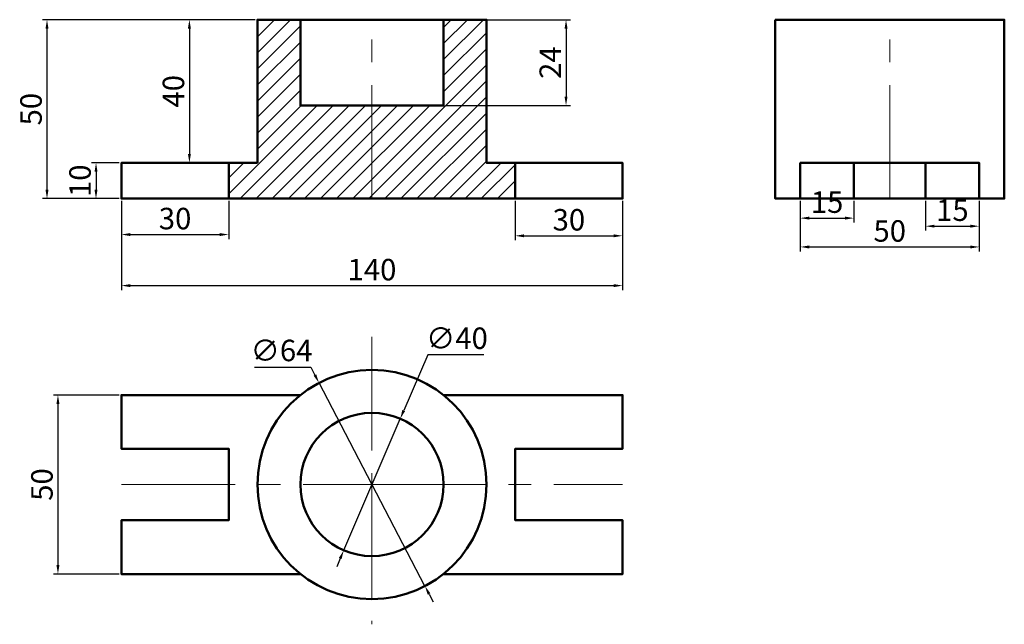
# Model space of a CAD drawing. Units: millimetres. Extents: x 177 to 452, y 51 to 220.
import ezdxf

# ---------------------------------------------------------------- set-up
doc = ezdxf.new("R2010")
doc.units = ezdxf.units.MM
doc.linetypes.add('CENTER', pattern=[50.8, 31.75, -6.35, 6.35, -6.35])
for name, color, linetype, lineweight in [('M-CNTR', 1, 'CENTER', 18), ('M-DIMS', 2, 'Continuous', 25), ('M-HATC', 8, 'Continuous', 18), ('M-OUTL', 7, 'Continuous', 50)]:
    doc.layers.add(name, color=color, linetype=linetype, lineweight=lineweight)
doc.styles.get("Standard").update_dxf_attribs({"font": 'arial.ttf'})
doc.dimstyles.new('ISO-25', dxfattribs={"dimtxt": 6, "dimasz": 2.5, "dimexe": 1.25, "dimexo": 0.625, "dimtad": 1, "dimtoh": 1, "dimdec": 1, "dimtxsty": 'Standard', "dimcen": 2.5, "dimadec": 0, "dimazin": 0, "dimtfac": 1, "dimtdec": 1, "dimtmove": 0, "dimatfit": 3, "dimfxl": 1, "dimarcsym": 0})

# ---------------------------------------------------------------- blocks, each defined once
blk = doc.blocks.new('*D1')
at = {"layer": 'Defpoints', "color": 0, "transparency": 16777216}
for p in [(295.75, 220.14), (295.75, 196.14), (329.95, 196.14)]:
    blk.add_point(p, dxfattribs=at)
at = {"layer": 'M-DIMS', "color": 0, "lineweight": -2, "transparency": 16777216}
for p, q in [((296.38, 220.14), (331.2, 220.14)), ((329.95, 217.64), (329.95, 198.64)), ((296.38, 196.14), (331.2, 196.14))]:
    blk.add_line(p, q, dxfattribs=at)
at = {"layer": 'M-DIMS', "color": 0, "transparency": 16777216}
for points in [[(329.54, 217.64), (330.37, 217.64), (329.95, 220.14)], [(329.54, 198.64), (330.37, 198.64), (329.95, 196.14)]]:
    blk.add_solid(points, dxfattribs=at)
at = {"layer": 'M-DIMS', "color": 0, "transparency": 16777216, "insert": (326.32, 208.14), "char_height": 6, "attachment_point": 5, "rotation": 90}
blk.add_mtext('24', dxfattribs=at)
blk = doc.blocks.new('*D2')
at = {"layer": 'Defpoints', "color": 0, "transparency": 16777216}
for p in [(205.75, 170.14), (235.75, 170.14), (235.75, 160.11)]:
    blk.add_point(p, dxfattribs=at)
at = {"layer": 'M-DIMS', "color": 0, "lineweight": -2, "transparency": 16777216}
for p, q in [((205.75, 169.51), (205.75, 158.86)), ((235.75, 169.51), (235.75, 158.86)), ((208.25, 160.11), (233.25, 160.11))]:
    blk.add_line(p, q, dxfattribs=at)
at = {"layer": 'M-DIMS', "color": 0, "transparency": 16777216}
for points in [[(208.25, 160.53), (208.25, 159.7), (205.75, 160.11)], [(233.25, 160.53), (233.25, 159.7), (235.75, 160.11)]]:
    blk.add_solid(points, dxfattribs=at)
at = {"layer": 'M-DIMS', "color": 0, "transparency": 16777216, "insert": (220.75, 163.8), "char_height": 6, "attachment_point": 5}
blk.add_mtext('30', dxfattribs=at)
blk = doc.blocks.new('*D3')
at = {"layer": 'Defpoints', "color": 0, "transparency": 16777216}
for p in [(315.75, 170.14), (345.75, 170.14), (345.75, 159.76)]:
    blk.add_point(p, dxfattribs=at)
at = {"layer": 'M-DIMS', "color": 0, "lineweight": -2, "transparency": 16777216}
for p, q in [((315.75, 169.51), (315.75, 158.51)), ((345.75, 169.51), (345.75, 158.51)), ((318.25, 159.76), (343.25, 159.76))]:
    blk.add_line(p, q, dxfattribs=at)
at = {"layer": 'M-DIMS', "color": 0, "transparency": 16777216}
for points in [[(318.25, 160.18), (318.25, 159.35), (315.75, 159.76)], [(343.25, 160.18), (343.25, 159.35), (345.75, 159.76)]]:
    blk.add_solid(points, dxfattribs=at)
at = {"layer": 'M-DIMS', "color": 0, "transparency": 16777216, "insert": (330.75, 163.46), "char_height": 6, "attachment_point": 5}
blk.add_mtext('30', dxfattribs=at)
blk = doc.blocks.new('*D4')
at = {"layer": 'Defpoints', "color": 0, "transparency": 16777216}
for p in [(205.75, 170.14), (345.75, 170.14), (345.75, 145.85)]:
    blk.add_point(p, dxfattribs=at)
at = {"layer": 'M-DIMS', "color": 0, "lineweight": -2, "transparency": 16777216}
for p, q in [((205.75, 169.51), (205.75, 144.6)), ((345.75, 169.51), (345.75, 144.6)), ((208.25, 145.85), (343.25, 145.85))]:
    blk.add_line(p, q, dxfattribs=at)
at = {"layer": 'M-DIMS', "color": 0, "transparency": 16777216}
for points in [[(208.25, 146.26), (208.25, 145.43), (205.75, 145.85)], [(343.25, 146.26), (343.25, 145.43), (345.75, 145.85)]]:
    blk.add_solid(points, dxfattribs=at)
at = {"layer": 'M-DIMS', "color": 0, "transparency": 16777216, "insert": (275.75, 149.53), "char_height": 6, "attachment_point": 5}
blk.add_mtext('140', dxfattribs=at)
blk = doc.blocks.new('*D5')
at = {"layer": 'Defpoints', "color": 0, "transparency": 16777216}
for p in [(205.75, 180.14), (198.67, 170.14), (205.75, 170.14)]:
    blk.add_point(p, dxfattribs=at)
at = {"layer": 'M-DIMS', "color": 0, "lineweight": -2, "transparency": 16777216}
for p, q in [((205.13, 180.14), (197.42, 180.14)), ((198.67, 177.64), (198.67, 172.64)), ((205.13, 170.14), (197.42, 170.14))]:
    blk.add_line(p, q, dxfattribs=at)
at = {"layer": 'M-DIMS', "color": 0, "transparency": 16777216}
for points in [[(198.25, 177.64), (199.08, 177.64), (198.67, 180.14)], [(198.25, 172.64), (199.08, 172.64), (198.67, 170.14)]]:
    blk.add_solid(points, dxfattribs=at)
at = {"layer": 'M-DIMS', "color": 0, "transparency": 16777216, "insert": (194.98, 175.14), "char_height": 6, "attachment_point": 5, "rotation": 90}
blk.add_mtext('10', dxfattribs=at)
blk = doc.blocks.new('*D6')
at = {"layer": 'Defpoints', "color": 0, "transparency": 16777216}
for p in [(243.75, 220.14), (224.75, 180.14), (243.75, 180.14)]:
    blk.add_point(p, dxfattribs=at)
at = {"layer": 'M-DIMS', "color": 0, "lineweight": -2, "transparency": 16777216}
for p, q in [((243.13, 220.14), (223.5, 220.14)), ((224.75, 217.64), (224.75, 182.64)), ((243.13, 180.14), (223.5, 180.14))]:
    blk.add_line(p, q, dxfattribs=at)
at = {"layer": 'M-DIMS', "color": 0, "transparency": 16777216}
for points in [[(224.34, 217.64), (225.17, 217.64), (224.75, 220.14)], [(224.34, 182.64), (225.17, 182.64), (224.75, 180.14)]]:
    blk.add_solid(points, dxfattribs=at)
at = {"layer": 'M-DIMS', "color": 0, "transparency": 16777216, "insert": (221.07, 200.14), "char_height": 6, "attachment_point": 5, "rotation": 90}
blk.add_mtext('40', dxfattribs=at)
blk = doc.blocks.new('*D7')
at = {"layer": 'Defpoints', "color": 0, "transparency": 16777216}
for p in [(243.75, 220.14), (184.97, 170.14), (205.75, 170.14)]:
    blk.add_point(p, dxfattribs=at)
at = {"layer": 'M-DIMS', "color": 0, "lineweight": -2, "transparency": 16777216}
for p, q in [((243.13, 220.14), (183.72, 220.14)), ((184.97, 217.64), (184.97, 172.64)), ((205.13, 170.14), (183.72, 170.14))]:
    blk.add_line(p, q, dxfattribs=at)
at = {"layer": 'M-DIMS', "color": 0, "transparency": 16777216}
for points in [[(184.56, 217.64), (185.39, 217.64), (184.97, 220.14)], [(184.56, 172.64), (185.39, 172.64), (184.97, 170.14)]]:
    blk.add_solid(points, dxfattribs=at)
at = {"layer": 'M-DIMS', "color": 0, "transparency": 16777216, "insert": (181.29, 195.14), "char_height": 6, "attachment_point": 5, "rotation": 90}
blk.add_mtext('50', dxfattribs=at)
blk = doc.blocks.new('*D8')
at = {"layer": 'Defpoints', "color": 0, "transparency": 16777216}
for p in [(395.37, 170.14), (445.37, 170.14), (445.37, 156.65)]:
    blk.add_point(p, dxfattribs=at)
at = {"layer": 'M-DIMS', "color": 0, "lineweight": -2, "transparency": 16777216}
for p, q in [((395.37, 169.51), (395.37, 155.4)), ((445.37, 169.51), (445.37, 155.4)), ((397.87, 156.65), (442.87, 156.65))]:
    blk.add_line(p, q, dxfattribs=at)
at = {"layer": 'M-DIMS', "color": 0, "transparency": 16777216}
for points in [[(397.87, 157.06), (397.87, 156.23), (395.37, 156.65)], [(442.87, 157.06), (442.87, 156.23), (445.37, 156.65)]]:
    blk.add_solid(points, dxfattribs=at)
at = {"layer": 'M-DIMS', "color": 0, "transparency": 16777216, "insert": (420.37, 160.34), "char_height": 6, "attachment_point": 5}
blk.add_mtext('50', dxfattribs=at)
blk = doc.blocks.new('*D9')
at = {"layer": 'Defpoints', "color": 0, "transparency": 16777216}
for p in [(395.37, 170.14), (410.37, 170.14), (410.37, 164.7)]:
    blk.add_point(p, dxfattribs=at)
at = {"layer": 'M-DIMS', "color": 0, "lineweight": -2, "transparency": 16777216}
for p, q in [((395.37, 169.51), (395.37, 163.45)), ((410.37, 169.51), (410.37, 163.45)), ((397.87, 164.7), (407.87, 164.7))]:
    blk.add_line(p, q, dxfattribs=at)
at = {"layer": 'M-DIMS', "color": 0, "transparency": 16777216}
for points in [[(397.87, 165.12), (397.87, 164.29), (395.37, 164.7)], [(407.87, 165.12), (407.87, 164.29), (410.37, 164.7)]]:
    blk.add_solid(points, dxfattribs=at)
at = {"layer": 'M-DIMS', "color": 0, "transparency": 16777216, "insert": (402.87, 168.39), "char_height": 6, "attachment_point": 5}
blk.add_mtext('15', dxfattribs=at)
blk = doc.blocks.new('*D10')
at = {"layer": 'Defpoints', "color": 0, "transparency": 16777216}
for p in [(430.37, 170.14), (445.37, 170.14), (445.37, 162.45)]:
    blk.add_point(p, dxfattribs=at)
at = {"layer": 'M-DIMS', "color": 0, "lineweight": -2, "transparency": 16777216}
for p, q in [((430.37, 169.51), (430.37, 161.2)), ((445.37, 169.51), (445.37, 161.2)), ((432.87, 162.45), (442.87, 162.45))]:
    blk.add_line(p, q, dxfattribs=at)
at = {"layer": 'M-DIMS', "color": 0, "transparency": 16777216}
for points in [[(432.87, 162.87), (432.87, 162.04), (430.37, 162.45)], [(442.87, 162.87), (442.87, 162.04), (445.37, 162.45)]]:
    blk.add_solid(points, dxfattribs=at)
at = {"layer": 'M-DIMS', "color": 0, "transparency": 16777216, "insert": (437.87, 166.14), "char_height": 6, "attachment_point": 5}
blk.add_mtext('15', dxfattribs=at)
blk = doc.blocks.new('*D11')
at = {"layer": 'Defpoints', "color": 0, "transparency": 16777216}
for p in [(260.96, 118.66), (290.55, 61.9)]:
    blk.add_point(p, dxfattribs=at)
at = {"layer": 'M-DIMS', "color": 0, "lineweight": -2, "transparency": 16777216}
for p, q in [((242.93, 123.09), (258.65, 123.09)), ((258.65, 123.09), (259.81, 120.87)), ((290.55, 61.9), (260.96, 118.66)), ((291.7, 59.69), (292.86, 57.47))]:
    blk.add_line(p, q, dxfattribs=at)
at = {"layer": 'M-DIMS', "color": 0, "transparency": 16777216}
for points in [[(260.18, 121.06), (259.44, 120.68), (260.96, 118.66)], [(292.07, 59.88), (291.33, 59.49), (290.55, 61.9)]]:
    blk.add_solid(points, dxfattribs=at)
at = {"layer": 'M-DIMS', "color": 0, "transparency": 16777216, "insert": (250.48, 126.95), "char_height": 6, "attachment_point": 5}
blk.add_mtext('∅64', dxfattribs=at)
blk = doc.blocks.new('*D12')
at = {"layer": 'Defpoints', "color": 0, "transparency": 16777216}
for p in [(283.64, 108.66), (267.87, 71.9)]:
    blk.add_point(p, dxfattribs=at)
at = {"layer": 'M-DIMS', "color": 0, "lineweight": -2, "transparency": 16777216}
for p, q in [((291.31, 126.52), (284.63, 110.96)), ((307.03, 126.52), (291.31, 126.52)), ((267.87, 71.9), (283.64, 108.66)), ((266.88, 69.6), (265.89, 67.31))]:
    blk.add_line(p, q, dxfattribs=at)
at = {"layer": 'M-DIMS', "color": 0, "transparency": 16777216}
for points in [[(284.24, 111.12), (285.01, 110.79), (283.64, 108.66)], [(266.5, 69.77), (267.26, 69.44), (267.87, 71.9)]]:
    blk.add_solid(points, dxfattribs=at)
at = {"layer": 'M-DIMS', "color": 0, "transparency": 16777216, "insert": (299.48, 130.37), "char_height": 6, "attachment_point": 5}
blk.add_mtext('∅40', dxfattribs=at)
blk = doc.blocks.new('*D13')
at = {"layer": 'Defpoints', "color": 0, "transparency": 16777216}
for p in [(205.75, 115.28), (188.03, 65.28), (205.75, 65.28)]:
    blk.add_point(p, dxfattribs=at)
at = {"layer": 'M-DIMS', "color": 0, "lineweight": -2, "transparency": 16777216}
for p, q in [((205.13, 115.28), (186.78, 115.28)), ((188.03, 112.78), (188.03, 67.78)), ((205.13, 65.28), (186.78, 65.28))]:
    blk.add_line(p, q, dxfattribs=at)
at = {"layer": 'M-DIMS', "color": 0, "transparency": 16777216}
for points in [[(187.61, 112.78), (188.45, 112.78), (188.03, 115.28)], [(187.61, 67.78), (188.45, 67.78), (188.03, 65.28)]]:
    blk.add_solid(points, dxfattribs=at)
at = {"layer": 'M-DIMS', "color": 0, "transparency": 16777216, "insert": (184.34, 90.28), "char_height": 6, "attachment_point": 5, "rotation": 90}
blk.add_mtext('50', dxfattribs=at)

msp = doc.modelspace()

# ---------------------------------------------------------------- hatches: boundary and pattern name
at = {"layer": 'M-HATC'}
h = msp.add_hatch(dxfattribs=at)
h.set_pattern_fill('ANSI31', color=256)
h.set_pattern_definition([(45, (166.474, 43.8026), (-2.245064, 2.245064), [])])
h.paths.add_polyline_path([(255.75, 220.14), (243.75, 220.14), (243.75, 180.14), (235.75, 180.14), (235.75, 170.14), (275.75, 170.14), (275.75, 196.14), (255.75, 196.14)])
h.paths.add_polyline_path([(315.75, 180.14), (307.75, 180.14), (307.75, 220.14), (295.75, 220.14), (295.75, 196.14), (275.75, 196.14), (275.75, 170.14), (315.75, 170.14)])

# ---------------------------------------------------------------- linework, layer by layer
at = {"layer": 'M-CNTR'}
for p, q in [((275.75, 170.14), (275.75, 220.14)), ((420.37, 170.14), (420.37, 220.14))]:
    msp.add_line(p, q, dxfattribs=at)
for points in [[(275.75, 131.53), (275.75, 90.28), (275.75, 51.23)], [(205.75, 90.28), (275.75, 90.28), (345.75, 90.28)]]:
    msp.add_lwpolyline(points, dxfattribs=at)
at = {"layer": 'M-OUTL'}
for p, q in [((235.75, 170.14), (235.75, 180.14)), ((315.75, 170.14), (315.75, 180.14)), ((410.37, 170.14), (410.37, 180.14)), ((430.37, 180.14), (430.37, 170.14))]:
    msp.add_line(p, q, dxfattribs=at)
for points in [[(243.75, 180.14), (243.75, 220.14), (307.75, 220.14), (307.75, 180.14), (345.75, 180.14), (345.75, 170.14), (205.75, 170.14), (205.75, 180.14)], [(388.37, 220.14), (452.37, 220.14), (452.37, 170.14), (388.37, 170.14)]]:
    msp.add_lwpolyline(points, close=True, dxfattribs=at)
for points in [[(255.75, 220.14), (255.75, 196.14), (295.75, 196.14), (295.75, 220.14)], [(445.37, 170.14), (445.37, 180.14), (395.37, 180.14), (395.37, 170.14)], [(255.78, 115.28), (205.75, 115.28), (205.75, 100.28), (235.75, 100.28), (235.75, 80.28), (205.75, 80.28), (205.75, 65.28), (255.78, 65.28)], [(295.73, 115.28), (345.75, 115.28), (345.75, 100.28), (315.75, 100.28), (315.75, 80.28), (345.75, 80.28), (345.75, 65.28), (295.73, 65.28)]]:
    msp.add_lwpolyline(points, dxfattribs=at)
for radius in [32, 20]:
    msp.add_circle((275.75, 90.28), radius, dxfattribs=at)

# ---------------------------------------------------------------- dimensions: what is measured, and where the dimension line sits
at = {"layer": 'M-DIMS'}
for base, p1, p2, picture, middle in [((184.97, 170.14), (243.75, 220.14), (205.75, 170.14), '*D7', (181.29, 195.14)), ((224.75, 180.14), (243.75, 220.14), (243.75, 180.14), '*D6', (221.07, 200.14)), ((329.95, 196.14), (295.75, 220.14), (295.75, 196.14), '*D1', (326.32, 208.14)), ((198.67, 170.14), (205.75, 180.14), (205.75, 170.14), '*D5', (194.98, 175.14)), ((188.03, 65.28), (205.75, 115.28), (205.75, 65.28), '*D13', (184.34, 90.28))]:
    dim = msp.add_linear_dim(base=base, p1=p1, p2=p2, angle=90, dimstyle='ISO-25', override={"dimclrd": 0, "dimclre": 0, "dimclrt": 0}, dxfattribs=at)
    dim.commit()
    dim.dimension.update_dxf_attribs({"geometry": picture, "text_midpoint": middle})
for base, p1, p2, picture, middle in [((410.37, 164.7), (395.37, 170.14), (410.37, 170.14), '*D9', (402.87, 168.39)), ((235.75, 160.11), (205.75, 170.14), (235.75, 170.14), '*D2', (220.75, 163.8)), ((345.75, 145.85), (205.75, 170.14), (345.75, 170.14), '*D4', (275.75, 149.53)), ((345.75, 159.76), (315.75, 170.14), (345.75, 170.14), '*D3', (330.75, 163.46)), ((445.37, 156.65), (395.37, 170.14), (445.37, 170.14), '*D8', (420.37, 160.34)), ((445.37, 162.45), (430.37, 170.14), (445.37, 170.14), '*D10', (437.87, 166.14))]:
    dim = msp.add_linear_dim(base=base, p1=p1, p2=p2, dimstyle='ISO-25', override={"dimclrd": 0, "dimclre": 0, "dimclrt": 0}, dxfattribs=at)
    dim.commit()
    dim.dimension.update_dxf_attribs({"geometry": picture, "text_midpoint": middle})
dim = msp.add_diameter_dim_2p(p1=(267.87, 71.9), p2=(283.64, 108.66), dimstyle='ISO-25', override={"dimclrd": 0, "dimclre": 0, "dimclrt": 0}, dxfattribs=at)
dim.commit()
dim.dimension.update_dxf_attribs({"geometry": '*D12', "text_midpoint": (299.48, 126.52), "dimtype": 163})
dim = msp.add_diameter_dim_2p(p1=(290.55, 61.9), p2=(260.96, 118.66), dimstyle='ISO-25', override={"dimclrd": 0, "dimclre": 0, "dimclrt": 0}, dxfattribs=at)
dim.commit()
dim.dimension.update_dxf_attribs({"geometry": '*D11', "text_midpoint": (250.48, 126.95)})

doc.saveas('drawing.dxf')
